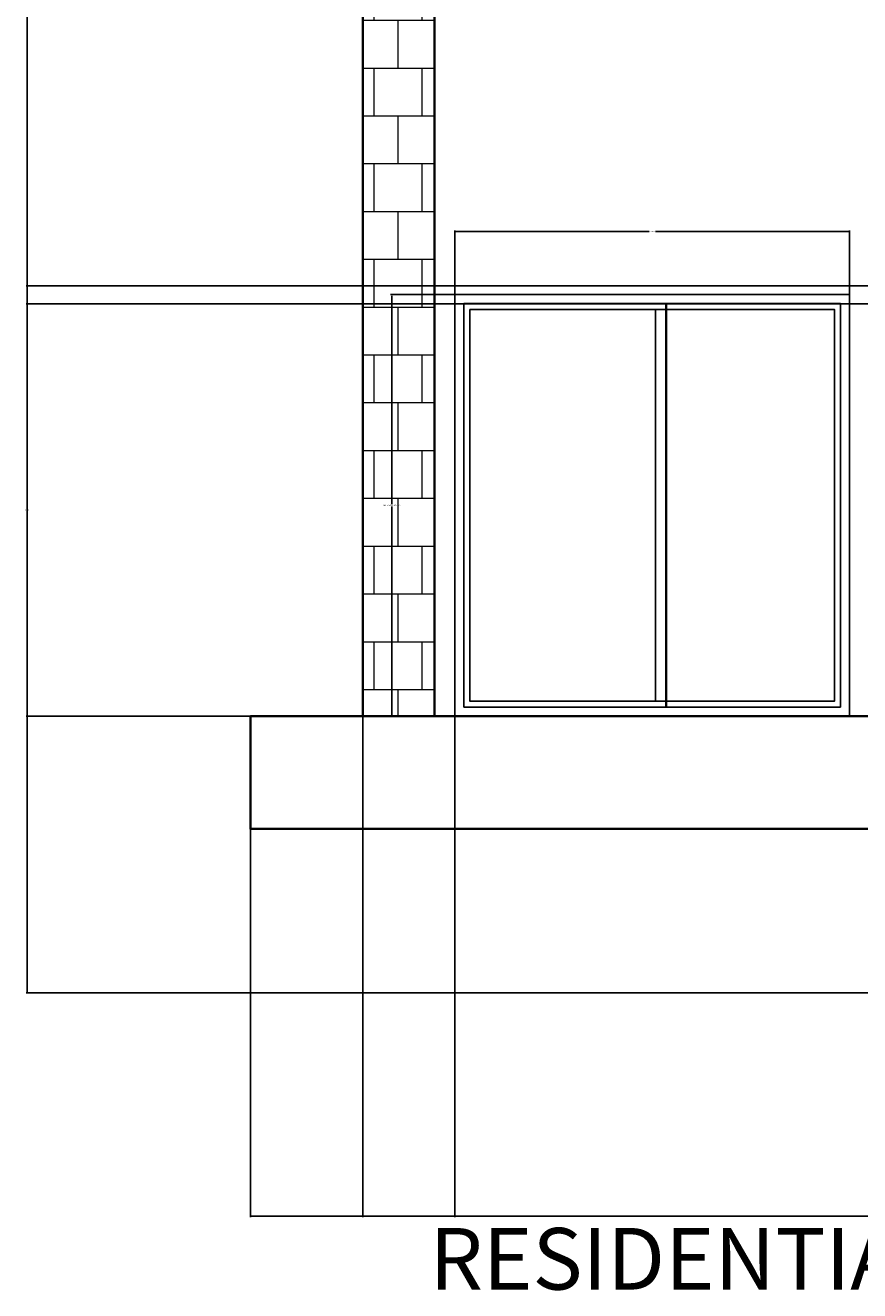
# Model space of a CAD drawing. Units: inches. Extents: x 10 to 404, y -77 to 696.
# Tile 1 of 5: x 10 to 149, y -77 to 135. Entities that reach past the tile are written whole.
import ezdxf

# ---------------------------------------------------------------- set-up
doc = ezdxf.new("R2010")
doc.units = ezdxf.units.IN
doc.header["$MEASUREMENT"] = 0
for name, color, linetype, lineweight in [('A-ANNO-DIMS', 2, 'Continuous', 18), ('A-ANNO-TEXT', 7, 'Continuous', 25), ('A-ELEV', 7, 'Continuous', 35), ('A-ELEV-PATT', 8, 'Continuous', 13), ('A-GLAZ', 4, 'Continuous', 25)]:
    doc.layers.add(name, color=color, linetype=linetype, lineweight=lineweight)
doc.styles.get("Standard").update_dxf_attribs({"font": 'arial.ttf'})
doc.dimstyles.get("Standard").update_dxf_attribs({"dimtxt": 0.18, "dimasz": 0.18, "dimexe": 0.18, "dimexo": 0.0625, "dimgap": 0.09, "dimtad": 0, "dimtih": 1, "dimtoh": 1, "dimdec": 4, "dimzin": 0, "dimdsep": 46, "dimtxsty": 'Standard', "dimcen": 0.09, "dimadec": 0, "dimazin": 0, "dimtfac": 1, "dimtdec": 4, "dimtofl": 0, "dimtmove": 0, "dimatfit": 3, "dimfxl": 1, "dimtolj": 1, "dimtzin": 0, "dimarcsym": 0})

# ---------------------------------------------------------------- blocks, each defined once
blk = doc.blocks.new('WIN-SLIDING-2P')
for p, q in [((83.01, 21.05), (83.01, 88.58)), ((83.01, 88.58), (105.51, 88.58)), ((105.51, 88.58), (146.03, 88.58)), ((146.03, 88.58), (146.03, 21.05)), ((105.51, 21.05), (83.01, 21.05)), ((146.03, 21.05), (105.51, 21.05))]:
    blk.add_line(p, q)
blk.add_lwpolyline([(81.51, 19.55), (81.51, 90.08), (147.53, 90.08), (147.53, 19.55)], close=True)
blk.add_lwpolyline([(115.07, 87.58), (115.07, 22.05), (84.01, 22.05), (84.01, 87.58), (104.51, 87.58)])
blk = doc.blocks.new('*D7')
at = {"layer": 'A-ANNO-DIMS', "color": 0, "lineweight": -2, "transparency": 16777216}
for p, q in [((81.44, 90.08), (70.75, 90.08)), ((70.93, 89.9), (70.93, 55)), ((70.93, 19.73), (70.93, 54.63)), ((81.44, 19.55), (70.75, 19.55))]:
    blk.add_line(p, q, dxfattribs=at)
at = {"layer": 'A-ANNO-DIMS', "color": 0, "transparency": 16777216}
for points in [[(70.9, 89.9), (70.96, 89.9), (70.93, 90.08)], [(70.9, 19.73), (70.96, 19.73), (70.93, 19.55)]]:
    blk.add_solid(points, dxfattribs=at)
at = {"layer": 'Defpoints', "color": 0, "transparency": 16777216}
for p in [(70.93, 90.08), (81.51, 90.08), (81.51, 19.55)]:
    blk.add_point(p, dxfattribs=at)
at = {"layer": 'A-ANNO-DIMS', "color": 0, "transparency": 16777216, "insert": (70.93, 54.82), "char_height": 0.18, "attachment_point": 5}
blk.add_mtext('\\A1;SLIDING WINDOW 71 TYP.', dxfattribs=at)
blk = doc.blocks.new('*D8')
at = {"layer": 'A-ANNO-DIMS', "color": 0, "lineweight": -2, "transparency": 16777216}
for p, q in [((81.51, 90.14), (81.51, 100.84)), ((81.69, 100.66), (113.99, 100.66)), ((147.35, 100.66), (115.05, 100.66)), ((147.53, 90.14), (147.53, 100.84))]:
    blk.add_line(p, q, dxfattribs=at)
at = {"layer": 'A-ANNO-DIMS', "color": 0, "transparency": 16777216}
for points in [[(81.69, 100.69), (81.69, 100.63), (81.51, 100.66)], [(147.35, 100.69), (147.35, 100.63), (147.53, 100.66)]]:
    blk.add_solid(points, dxfattribs=at)
at = {"layer": 'Defpoints', "color": 0, "transparency": 16777216}
for p in [(147.53, 100.66), (81.51, 90.08), (147.53, 90.08)]:
    blk.add_point(p, dxfattribs=at)
at = {"layer": 'A-ANNO-DIMS', "color": 0, "transparency": 16777216, "insert": (114.52, 100.66), "char_height": 0.18, "attachment_point": 5}
blk.add_mtext('\\A1;66 TYP.', dxfattribs=at)
blk = doc.blocks.new('*D9')
at = {"layer": 'A-ANNO-DIMS', "color": 0, "lineweight": -2, "transparency": 16777216}
for p, q in [((47.29, 0.6), (47.29, -64.31)), ((365.94, 0.6), (365.94, -64.31)), ((47.47, -64.13), (206.15, -64.13)), ((365.76, -64.13), (207.08, -64.13))]:
    blk.add_line(p, q, dxfattribs=at)
at = {"layer": 'A-ANNO-DIMS', "color": 0, "transparency": 16777216}
for points in [[(47.47, -64.1), (47.47, -64.16), (47.29, -64.13)], [(365.76, -64.1), (365.76, -64.16), (365.94, -64.13)]]:
    blk.add_solid(points, dxfattribs=at)
at = {"layer": 'Defpoints', "color": 0, "transparency": 16777216}
for p in [(47.29, 0.67), (365.94, 0.67), (365.94, -64.13)]:
    blk.add_point(p, dxfattribs=at)
at = {"layer": 'A-ANNO-DIMS', "color": 0, "transparency": 16777216, "insert": (206.61, -64.13), "char_height": 0.18, "attachment_point": 5}
blk.add_mtext('\\A1;318.65', dxfattribs=at)
blk = doc.blocks.new('*D10')
at = {"layer": 'A-ANNO-DIMS', "color": 0, "lineweight": -2, "transparency": 16777216}
for p, q in [((65.94, 657.96), (9.76, 657.96)), ((9.94, 657.78), (9.94, 315.77)), ((9.94, -26.6), (9.94, 315.41)), ((176.46, -26.78), (9.76, -26.78))]:
    blk.add_line(p, q, dxfattribs=at)
at = {"layer": 'A-ANNO-DIMS', "color": 0, "transparency": 16777216}
for points in [[(9.91, 657.78), (9.97, 657.78), (9.94, 657.96)], [(9.91, -26.6), (9.97, -26.6), (9.94, -26.78)]]:
    blk.add_solid(points, dxfattribs=at)
at = {"layer": 'Defpoints', "color": 0, "transparency": 16777216}
for p in [(9.94, 657.96), (66.01, 657.96), (176.53, -26.78)]:
    blk.add_point(p, dxfattribs=at)
at = {"layer": 'A-ANNO-DIMS', "color": 0, "transparency": 16777216, "insert": (9.94, 315.59), "char_height": 0.18, "attachment_point": 5}
blk.add_mtext('\\A1;684.7', dxfattribs=at)
blk = doc.blocks.new('*D11')
at = {"layer": 'A-ANNO-DIMS', "color": 0, "lineweight": -2, "transparency": 16777216}
for p, q in [((47.29, 19.49), (47.29, -64.31)), ((66.1, 19.49), (66.1, -64.31)), ((47.47, -64.13), (56.33, -64.13)), ((65.92, -64.13), (57.06, -64.13))]:
    blk.add_line(p, q, dxfattribs=at)
at = {"layer": 'A-ANNO-DIMS', "color": 0, "transparency": 16777216}
for points in [[(47.47, -64.1), (47.47, -64.16), (47.29, -64.13)], [(65.92, -64.1), (65.92, -64.16), (66.1, -64.13)]]:
    blk.add_solid(points, dxfattribs=at)
at = {"layer": 'Defpoints', "color": 0, "transparency": 16777216}
for p in [(47.29, 19.55), (66.1, 19.55), (66.1, -64.13)]:
    blk.add_point(p, dxfattribs=at)
at = {"layer": 'A-ANNO-DIMS', "color": 0, "transparency": 16777216, "insert": (56.7, -64.13), "char_height": 0.18, "attachment_point": 5}
blk.add_mtext('\\A1;18.81', dxfattribs=at)
blk = doc.blocks.new('*D12')
at = {"layer": 'A-ANNO-DIMS', "color": 0, "lineweight": -2, "transparency": 16777216}
for p, q in [((66.1, 19.49), (66.1, -64.31)), ((81.51, 19.49), (81.51, -64.31)), ((66.28, -64.13), (73.35, -64.13)), ((81.33, -64.13), (74.26, -64.13))]:
    blk.add_line(p, q, dxfattribs=at)
at = {"layer": 'A-ANNO-DIMS', "color": 0, "transparency": 16777216}
for points in [[(66.28, -64.1), (66.28, -64.16), (66.1, -64.13)], [(81.33, -64.1), (81.33, -64.16), (81.51, -64.13)]]:
    blk.add_solid(points, dxfattribs=at)
at = {"layer": 'Defpoints', "color": 0, "transparency": 16777216}
for p in [(66.1, 19.55), (81.51, 19.55), (81.51, -64.13)]:
    blk.add_point(p, dxfattribs=at)
at = {"layer": 'A-ANNO-DIMS', "color": 0, "transparency": 16777216, "insert": (73.8, -64.13), "char_height": 0.18, "attachment_point": 5}
blk.add_mtext('\\A1;15.404', dxfattribs=at)
blk = doc.blocks.new('*D13')
at = {"layer": 'A-ANNO-DIMS', "color": 0, "lineweight": -2, "transparency": 16777216}
for p, q in [((81.51, 19.49), (81.51, -64.31)), ((167.67, 19.49), (167.67, -64.31)), ((81.69, -64.13), (124.19, -64.13)), ((167.49, -64.13), (124.98, -64.13))]:
    blk.add_line(p, q, dxfattribs=at)
at = {"layer": 'A-ANNO-DIMS', "color": 0, "transparency": 16777216}
for points in [[(81.69, -64.1), (81.69, -64.16), (81.51, -64.13)], [(167.49, -64.1), (167.49, -64.16), (167.67, -64.13)]]:
    blk.add_solid(points, dxfattribs=at)
at = {"layer": 'Defpoints', "color": 0, "transparency": 16777216}
for p in [(81.51, 19.55), (167.67, 19.55), (167.67, -64.13)]:
    blk.add_point(p, dxfattribs=at)
at = {"layer": 'A-ANNO-DIMS', "color": 0, "transparency": 16777216, "insert": (124.59, -64.13), "char_height": 0.18, "attachment_point": 5}
blk.add_mtext('\\A1;86.16', dxfattribs=at)
blk = doc.blocks.new('*D54')
at = {"layer": 'A-ANNO-DIMS', "color": 0, "lineweight": -2, "transparency": 16777216}
for p, q in [((167.6, 91.55), (9.76, 91.55)), ((9.94, 91.37), (9.94, 55.73)), ((9.94, 19.73), (9.94, 55.37)), ((167.6, 19.55), (9.76, 19.55))]:
    blk.add_line(p, q, dxfattribs=at)
at = {"layer": 'A-ANNO-DIMS', "color": 0, "transparency": 16777216}
for points in [[(9.91, 91.37), (9.97, 91.37), (9.94, 91.55)], [(9.91, 19.73), (9.97, 19.73), (9.94, 19.55)]]:
    blk.add_solid(points, dxfattribs=at)
at = {"layer": 'Defpoints', "color": 0, "transparency": 16777216}
for p in [(9.94, 91.55), (167.67, 91.55), (167.67, 19.55)]:
    blk.add_point(p, dxfattribs=at)
at = {"layer": 'A-ANNO-DIMS', "color": 0, "transparency": 16777216, "insert": (9.94, 55.55), "char_height": 0.18, "attachment_point": 5}
blk.add_mtext('\\A1;72', dxfattribs=at)
blk = doc.blocks.new('*D55')
at = {"layer": 'A-ANNO-DIMS', "color": 0, "lineweight": -2, "transparency": 16777216}
for p, q in [((170.6, 88.53), (9.76, 88.53)), ((9.94, 88.35), (9.94, 54.22)), ((9.94, 19.73), (9.94, 53.86)), ((170.6, 19.55), (9.76, 19.55))]:
    blk.add_line(p, q, dxfattribs=at)
at = {"layer": 'A-ANNO-DIMS', "color": 0, "transparency": 16777216}
for points in [[(9.91, 88.35), (9.97, 88.35), (9.94, 88.53)], [(9.91, 19.73), (9.97, 19.73), (9.94, 19.55)]]:
    blk.add_solid(points, dxfattribs=at)
at = {"layer": 'Defpoints', "color": 0, "transparency": 16777216}
for p in [(9.94, 88.53), (170.67, 88.53), (170.67, 19.55)]:
    blk.add_point(p, dxfattribs=at)
at = {"layer": 'A-ANNO-DIMS', "color": 0, "transparency": 16777216, "insert": (9.94, 54.04), "char_height": 0.18, "attachment_point": 5}
blk.add_mtext('\\A1;68.98', dxfattribs=at)

msp = doc.modelspace()

# ---------------------------------------------------------------- hatches: boundary and pattern name
at = {"layer": 'A-ELEV-PATT'}
h = msp.add_hatch(dxfattribs=at)
h.set_pattern_fill('AR-B88', color=256)
h.paths.add_polyline_path([(78.1013, 499.5535), (66.1013, 499.5535), (66.1013, 19.5535), (78.1013, 19.5535)])

# ---------------------------------------------------------------- linework, layer by layer
at = {"layer": 'A-ELEV'}
for p, q in [((66.1013, 619.5535), (66.1013, 19.5535)), ((78.1013, 619.5535), (78.1013, 19.5535)), ((116.8527, 21.0535), (116.8527, 88.5811)), ((66.1013, 19.5535), (341.8668, 19.5535))]:
    msp.add_line(p, q, dxfattribs=at)
msp.add_lwpolyline([(47.2905, 19.5535), (365.9356, 19.5535), (365.9356, 0.6668), (47.2905, 0.6668)], close=True, dxfattribs=at)
at = {"layer": 'A-GLAZ'}
msp.add_lwpolyline([(84.0054, 87.5811), (145.0304, 87.5811), (145.0304, 22.0535), (105.5054, 22.0535)], dxfattribs=at)

# ---------------------------------------------------------------- block references
msp.add_blockref('WIN-SLIDING-2P', (0, 0), dxfattribs=at)

# ---------------------------------------------------------------- texts
at = {"layer": 'A-ANNO-TEXT'}
msp.add_text('RESIDENTIAL BUILDING G+4 ELEVATION', height=10.308105, dxfattribs=at).set_placement((77.2746, -76.4214))

# ---------------------------------------------------------------- dimensions: what is measured, and where the dimension line sits
at = {"layer": 'A-ANNO-DIMS'}
for base, p1, p2, override, picture, middle in [((9.9405, 657.9612), (176.5266, -26.7816), (66.0062, 657.9612), {"dimdec": 1, "dimlfac": 1, "dimrnd": 0, "dimzin": 0, "dimdsep": 46, "dimlunit": 2}, '*D10', (9.9405, 315.5898)), ((9.9405, 91.5535), (167.6671, 19.5535), (167.6671, 91.5535), {"dimdec": 0, "dimlfac": 1, "dimrnd": 0, "dimzin": 0, "dimdsep": 46, "dimlunit": 2}, '*D54', (9.9405, 55.5535)), ((9.9405, 88.5306), (170.6671, 19.5535), (170.6671, 88.5306), {"dimdec": 2, "dimlfac": 1, "dimrnd": 0, "dimzin": 0, "dimdsep": 46, "dimlunit": 2}, '*D55', (9.9405, 54.0421))]:
    dim = msp.add_linear_dim(base=base, p1=p1, p2=p2, angle=90, dimstyle='Standard', override=override, dxfattribs=at)
    dim.commit()
    dim.dimension.update_dxf_attribs({"geometry": picture, "text_midpoint": middle})
dim = msp.add_linear_dim(base=(147.5304, 100.6603), p1=(81.5054, 90.0811), p2=(147.5304, 90.0811), text='<> TYP.', dimstyle='Standard', override={"dimdec": 0, "dimlfac": 1, "dimrnd": 0, "dimzin": 0, "dimdsep": 46, "dimlunit": 2}, dxfattribs=at)
dim.commit()
dim.dimension.update_dxf_attribs({"geometry": '*D8', "text_midpoint": (114.5179, 100.6603)})
dim = msp.add_linear_dim(base=(70.9263, 90.0811), p1=(81.5054, 19.5535), p2=(81.5054, 90.0811), angle=90, text='SLIDING WINDOW <> TYP.', dimstyle='Standard', override={"dimdec": 0, "dimlfac": 1, "dimrnd": 0, "dimzin": 0, "dimdsep": 46, "dimlunit": 2}, dxfattribs=at)
dim.commit()
dim.dimension.update_dxf_attribs({"geometry": '*D7', "text_midpoint": (70.9263, 54.8173)})
for base, p1, p2, override, picture, middle in [((66.1013, -64.1316), (47.2905, 19.5535), (66.1013, 19.5535), {"dimdec": 2, "dimlfac": 1, "dimrnd": 0, "dimzin": 0, "dimdsep": 46, "dimlunit": 2}, '*D11', (56.6959, -64.1316)), ((81.5054, -64.1316), (66.1013, 19.5535), (81.5054, 19.5535), {"dimdec": 3, "dimlfac": 1, "dimrnd": 0, "dimzin": 0, "dimdsep": 46, "dimlunit": 2}, '*D12', (73.8034, -64.1316)), ((167.6671, -64.1316), (81.5054, 19.5535), (167.6671, 19.5535), {"dimdec": 2, "dimlfac": 1, "dimrnd": 0, "dimzin": 0, "dimdsep": 46, "dimlunit": 2}, '*D13', (124.5863, -64.1316)), ((365.9356, -64.1316), (47.2905, 0.6668), (365.9356, 0.6668), {"dimdec": 2, "dimlfac": 1, "dimrnd": 0, "dimzin": 0, "dimdsep": 46, "dimlunit": 2}, '*D9', (206.6131, -64.1316))]:
    dim = msp.add_linear_dim(base=base, p1=p1, p2=p2, dimstyle='Standard', override=override, dxfattribs=at)
    dim.commit()
    dim.dimension.update_dxf_attribs({"geometry": picture, "text_midpoint": middle})

doc.saveas('drawing.dxf')
